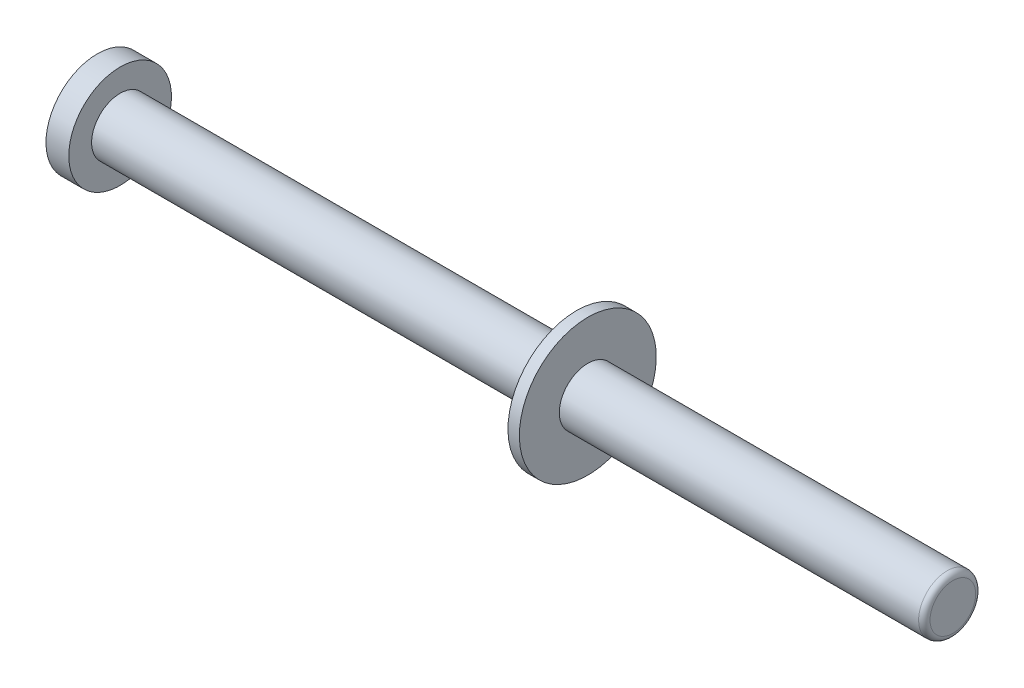
from build123d import *

# Parameters (mm, degrees)
EDGE_FILLET_R1_R = 1


with BuildPart() as part:
    # Shaft Profile Sketch → Shaft Body Revolve (revolve)
    with BuildSketch(Plane.XY):
        Polygon((-150, 0), (-150, 9), (-146, 9), (-146, 5), (-66, 5), (-66, 12), (-64, 12), (-64, 5), (0, 5), (0, 0), align=None)
    revolve(axis=Axis((0, 0, 0), (-1, 0, 0)))

    # Edge Fillet R1
    edge_fillet_r1_edges = [part.edges().sort_by_distance(p)[0] for p in [
        (0, -5, 0),
    ]]
    fillet(edge_fillet_r1_edges, radius=EDGE_FILLET_R1_R)


solid = part.part
